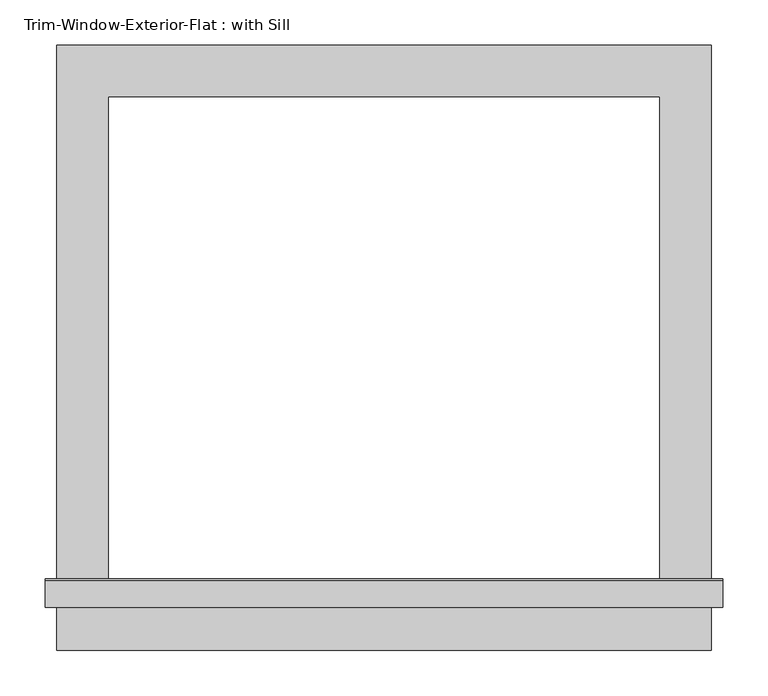
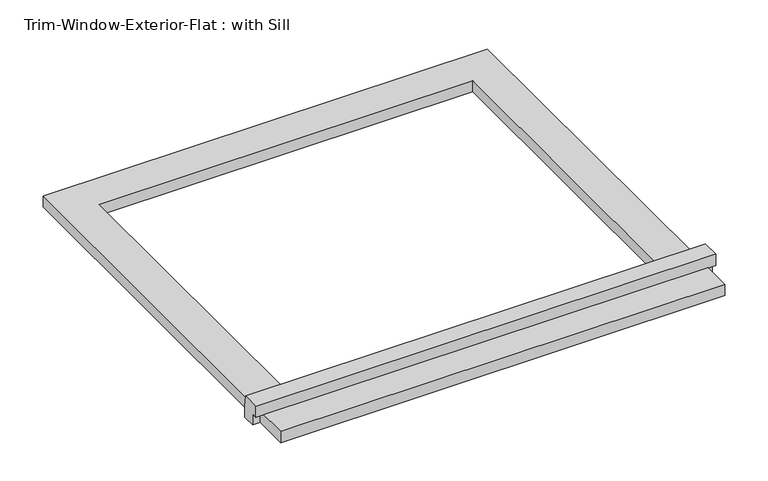
"""IFC4 building model written with IfcOpenShell, lengths in millimetres: proxy geometry, Trim-Window-Exterior-Flat : with Sill."""

from ifc_helpers import new_model, si_unit, frame, origin, origin_with_axes, place, context, project, spatial, polyline, outline, extrude, source, transform, mapped, element, save


def trim_window_exterior_flat_with_sill_e6f34eb5(model_context):
    return source(origin(), model_context, "Body", "SweptSolid", [
        extrude(outline(polyline([(361.95, -555.5823709), (361.95, -612.7323709), (-361.95, -612.7323709), (-361.95, -555.5823709), (361.95, -555.5823709)])), origin_with_axes(), (0.0, 0.0, 1.0), 19.05),
        extrude(outline(polyline([(-565.15, 38.1), (-535.8580645, 38.1), (-533.4, 19.05), (-533.4, 0.0), (-555.5823709, 0.0), (-555.5823709, 19.05), (-565.15, 19.05), (-565.15, 38.1)])), frame((-374.65, 0.0, 0.0), z_axis=(1.0, 0.0, 0.0), x_axis=(0.0, 1.0, 0.0)), (0.0, 0.0, 1.0), 749.3),
        extrude(outline(polyline([(-361.95, 57.15), (361.95, 57.15), (361.95, -533.4), (304.8, -533.4), (304.8, 0.0), (-304.8, 0.0), (-304.8, -533.4), (-361.95, -533.4), (-361.95, 57.15)])), origin_with_axes(), (0.0, 0.0, 1.0), 19.05),
    ])


if __name__ == "__main__":
    model = new_model("IFC4")
    model_context = context("Model", 3, world=origin())
    ifc_project = project(units=[si_unit("LENGTHUNIT", "METRE", prefix="MILLI")], contexts=[model_context])
    site = spatial("IfcSite", under=ifc_project)
    building = spatial("IfcBuilding", under=site)
    placement = place(None, origin())
    trim_window_exterior_flat_with_sill_shape = trim_window_exterior_flat_with_sill_e6f34eb5(model_context)
    element("IfcBuildingElementProxy", 1, Name="Trim-Window-Exterior-Flat : with Sill", ObjectType="Trim-Window-Exterior-Flat : with Sill", at=placement, inside=building, context=model_context, shape_type="MappedRepresentation", body=[
        mapped(trim_window_exterior_flat_with_sill_shape, transform((0.0, 0.0, 0.0), x_axis=(1.0, 0.0, 0.0), y_axis=(0.0, 1.0, 0.0), z_axis=(0.0, 0.0, 1.0))),
    ])
    save(model, "model.ifc")

# Revit data of these elements
# Type "Trim-Window-Exterior-Flat : with Sill"
#   Trim Width = 0' - 2 1/4"
#   Trim Thickness_Picture Frame = 0' - 1 1/4"
#   Trim Thickness_with Sill = 0' - 0 3/4"
#   Sill Thickness = 0' - 1 1/4"
#   Opening Width [instance default] = 2' - 0"
#   Opening Height [instance default] = 3' - 0"
#   Default Elevation = 4' - 0"
#   Sill = yes
#   Picture Frame = no
#   Trim Material [instance default] = none
# Element 1 (IfcBuildingElementProxy, "Trim-Window-Exterior-Flat : with Sill")
#   Opening Height = 1' - 9"
#   Trim Material = Clad - White
#   Materials on its faces: "Clad - White"
# Materials
#   "Clad - White": class "Wood", colour RGB 242 242 238, transparency 0, Cost = 0
